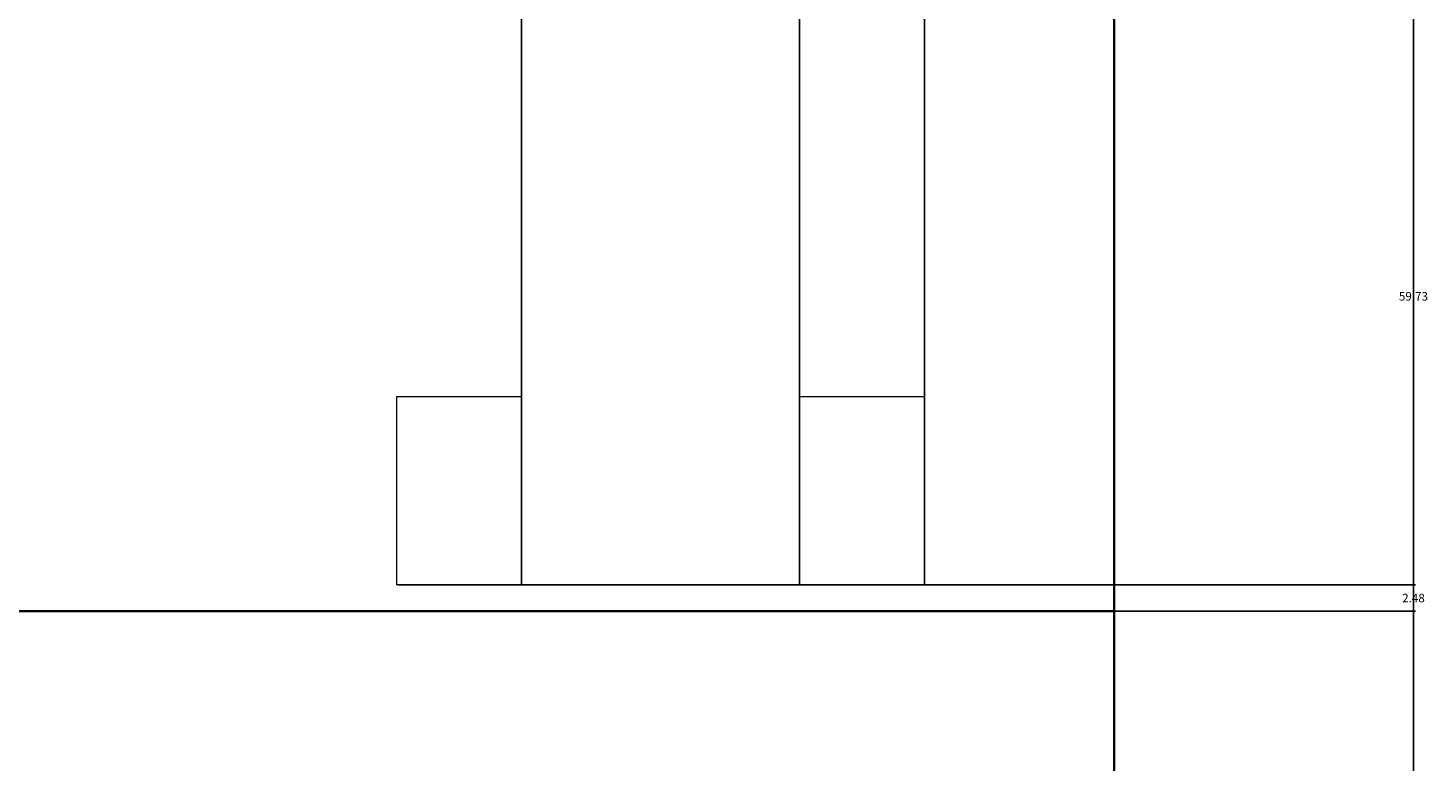
# Model space of a CAD drawing. Units: inches. Extents: x 69 to 650, y -16 to 573.
# Tile 25 of 26: x 516 to 649, y 398 to 467. Entities that reach past the tile are written whole.
import ezdxf

# ---------------------------------------------------------------- set-up
doc = ezdxf.new("R2010")
doc.units = ezdxf.units.IN
doc.header["$MEASUREMENT"] = 0
for name, color, linetype, lineweight in [('A-ANNO-DIMS', 2, 'Continuous', 18), ('A-GLAZ', 4, 'Continuous', 18), ('A-WALL', 7, 'Continuous', 35)]:
    doc.layers.add(name, color=color, linetype=linetype, lineweight=lineweight)
doc.styles.get("Standard").update_dxf_attribs({"font": 'arial.ttf'})
doc.dimstyles.get("Standard").update_dxf_attribs({"dimtxt": 0.8125, "dimasz": 0.18, "dimexe": 0.18, "dimexo": 0.0625, "dimgap": 0.09, "dimtad": 0, "dimtih": 1, "dimtoh": 1, "dimdec": 4, "dimzin": 0, "dimdsep": 46, "dimlunit": 4, "dimtxsty": 'Standard', "dimcen": 0.09, "dimadec": 0, "dimazin": 0, "dimtfac": 1, "dimtdec": 4, "dimtofl": 0, "dimtmove": 0, "dimatfit": 3, "dimfxl": 1, "dimtolj": 1, "dimtzin": 0, "dimarcsym": 0})

# ---------------------------------------------------------------- blocks, each defined once
blk = doc.blocks.new('WIN-UPPER-SMALL')
blk.add_lwpolyline([(0, 17.88), (11.84, 17.88), (11.84, 0), (0, 0)], close=True)
blk = doc.blocks.new('*D19')
at = {"layer": 'A-ANNO-DIMS', "color": 0, "lineweight": -2, "transparency": 16777216}
for p, q in [((99.56, 471.72), (99.56, 572.74)), ((619.56, 87.99), (619.56, 572.74)), ((99.74, 572.56), (358.57, 572.56)), ((619.38, 572.56), (360.54, 572.56))]:
    blk.add_line(p, q, dxfattribs=at)
at = {"layer": 'A-ANNO-DIMS', "color": 0, "transparency": 16777216}
for points in [[(99.74, 572.59), (99.74, 572.53), (99.56, 572.56)], [(619.38, 572.59), (619.38, 572.53), (619.56, 572.56)]]:
    blk.add_solid(points, dxfattribs=at)
at = {"layer": 'Defpoints', "color": 0, "transparency": 16777216}
for p in [(619.56, 572.56), (99.56, 471.66), (619.56, 87.93)]:
    blk.add_point(p, dxfattribs=at)
at = {"layer": 'A-ANNO-DIMS', "color": 0, "transparency": 16777216, "insert": (359.56, 572.56), "char_height": 0.812, "attachment_point": 5}
blk.add_mtext('\\A1;520', dxfattribs=at)
blk = doc.blocks.new('*D20')
at = {"layer": 'A-ANNO-DIMS', "color": 0, "lineweight": -2, "transparency": 16777216}
for p, q in [((504.24, 544.16), (648.14, 544.16)), ((647.96, 543.98), (647.96, 304.55)), ((647.96, 64.11), (647.96, 303.54)), ((619.62, 63.93), (648.14, 63.93))]:
    blk.add_line(p, q, dxfattribs=at)
at = {"layer": 'A-ANNO-DIMS', "color": 0, "transparency": 16777216}
for points in [[(647.93, 543.98), (647.99, 543.98), (647.96, 544.16)], [(647.93, 64.11), (647.99, 64.11), (647.96, 63.93)]]:
    blk.add_solid(points, dxfattribs=at)
at = {"layer": 'Defpoints', "color": 0, "transparency": 16777216}
for p in [(504.18, 544.16), (647.96, 544.16), (619.56, 63.93)]:
    blk.add_point(p, dxfattribs=at)
at = {"layer": 'A-ANNO-DIMS', "color": 0, "transparency": 16777216, "insert": (647.96, 304.04), "char_height": 0.812, "attachment_point": 5}
blk.add_mtext('\\A1;480.2', dxfattribs=at)
blk = doc.blocks.new('*D48')
at = {"layer": 'A-ANNO-DIMS', "color": 0, "lineweight": -2, "transparency": 16777216}
for p, q in [((619.62, 471.66), (648.14, 471.66)), ((647.96, 471.48), (647.96, 442.3)), ((647.96, 412.11), (647.96, 441.29)), ((619.62, 411.93), (648.14, 411.93))]:
    blk.add_line(p, q, dxfattribs=at)
at = {"layer": 'A-ANNO-DIMS', "color": 0, "transparency": 16777216}
for points in [[(647.93, 471.48), (647.99, 471.48), (647.96, 471.66)], [(647.93, 412.11), (647.99, 412.11), (647.96, 411.93)]]:
    blk.add_solid(points, dxfattribs=at)
at = {"layer": 'Defpoints', "color": 0, "transparency": 16777216}
for p in [(619.56, 471.66), (647.96, 471.66), (619.56, 411.93)]:
    blk.add_point(p, dxfattribs=at)
at = {"layer": 'A-ANNO-DIMS', "color": 0, "transparency": 16777216, "insert": (647.96, 441.79), "char_height": 0.812, "attachment_point": 5}
blk.add_mtext('\\A1;59.73', dxfattribs=at)
blk = doc.blocks.new('*D55')
at = {"layer": 'A-ANNO-DIMS', "color": 0, "lineweight": -2, "transparency": 16777216}
for p, q in [((563.31, 414.48), (563.31, 572.74)), ((589.7, 414.48), (589.7, 572.74)), ((563.49, 572.56), (575.03, 572.56)), ((589.52, 572.56), (577.97, 572.56))]:
    blk.add_line(p, q, dxfattribs=at)
at = {"layer": 'A-ANNO-DIMS', "color": 0, "transparency": 16777216}
for points in [[(563.49, 572.59), (563.49, 572.53), (563.31, 572.56)], [(589.52, 572.59), (589.52, 572.53), (589.7, 572.56)]]:
    blk.add_solid(points, dxfattribs=at)
at = {"layer": 'Defpoints', "color": 0, "transparency": 16777216}
for p in [(589.7, 572.56), (563.31, 414.41), (589.7, 414.41)]:
    blk.add_point(p, dxfattribs=at)
at = {"layer": 'A-ANNO-DIMS', "color": 0, "transparency": 16777216, "insert": (576.5, 572.56), "char_height": 0.812, "attachment_point": 5}
blk.add_mtext('\\A1;26.39', dxfattribs=at)
blk = doc.blocks.new('*D56')
at = {"layer": 'A-ANNO-DIMS', "color": 0, "lineweight": -2, "transparency": 16777216}
for p, q in [((601.54, 414.48), (601.54, 572.74)), ((619.56, 411.99), (619.56, 572.74)), ((601.72, 572.56), (608.81, 572.56)), ((619.38, 572.56), (612.29, 572.56))]:
    blk.add_line(p, q, dxfattribs=at)
at = {"layer": 'A-ANNO-DIMS', "color": 0, "transparency": 16777216}
for points in [[(601.72, 572.59), (601.72, 572.53), (601.54, 572.56)], [(619.38, 572.59), (619.38, 572.53), (619.56, 572.56)]]:
    blk.add_solid(points, dxfattribs=at)
at = {"layer": 'Defpoints', "color": 0, "transparency": 16777216}
for p in [(619.56, 572.56), (601.54, 414.41), (619.56, 411.93)]:
    blk.add_point(p, dxfattribs=at)
at = {"layer": 'A-ANNO-DIMS', "color": 0, "transparency": 16777216, "insert": (610.55, 572.56), "char_height": 0.812, "attachment_point": 5}
blk.add_mtext('\\A1;18.018', dxfattribs=at)
blk = doc.blocks.new('*D57')
at = {"layer": 'A-ANNO-DIMS', "color": 0, "lineweight": -2, "transparency": 16777216}
for p, q in [((551.53, 414.41), (648.14, 414.41)), ((647.96, 414.23), (647.96, 413.68)), ((500.33, 411.93), (648.14, 411.93)), ((647.96, 412.11), (647.96, 412.67))]:
    blk.add_line(p, q, dxfattribs=at)
at = {"layer": 'A-ANNO-DIMS', "color": 0, "transparency": 16777216}
for points in [[(647.93, 414.23), (647.99, 414.23), (647.96, 414.41)], [(647.93, 412.11), (647.99, 412.11), (647.96, 411.93)]]:
    blk.add_solid(points, dxfattribs=at)
at = {"layer": 'Defpoints', "color": 0, "transparency": 16777216}
for p in [(551.46, 414.41), (500.26, 411.93), (647.96, 411.93)]:
    blk.add_point(p, dxfattribs=at)
at = {"layer": 'A-ANNO-DIMS', "color": 0, "transparency": 16777216, "insert": (647.96, 413.17), "char_height": 0.812, "attachment_point": 5}
blk.add_mtext('\\A1;2.48', dxfattribs=at)

msp = doc.modelspace()

# ---------------------------------------------------------------- linework, layer by layer
at = {"layer": 'A-WALL'}
for p, q in [((619.555, 411.93), (619.555, 471.6595)), ((99.556, 411.93), (619.555, 411.93)), ((619.555, 411.93), (619.555, 69.3788))]:
    msp.add_line(p, q, dxfattribs=at)

# ---------------------------------------------------------------- block references
at = {"layer": 'A-GLAZ'}
for p in [(551.4642, 414.415), (589.6959, 414.415)]:
    msp.add_blockref('WIN-UPPER-SMALL', p, dxfattribs=at)

# ---------------------------------------------------------------- dimensions: what is measured, and where the dimension line sits
at = {"layer": 'A-ANNO-DIMS'}
for base, p1, p2, override, picture, middle in [((619.555, 572.5573), (99.556, 471.6595), (619.555, 87.93), {"dimdec": 0, "dimlfac": 1, "dimrnd": 0, "dimzin": 0, "dimdsep": 46, "dimlunit": 2}, '*D19', (359.5555, 572.5573)), ((589.6958, 572.5573), (563.3054, 414.4146), (589.6958, 414.4146), {"dimdec": 2, "dimlfac": 1, "dimrnd": 0, "dimzin": 0, "dimdsep": 46, "dimlunit": 2}, '*D55', (576.5006, 572.5573)), ((619.555, 572.5573), (601.5371, 414.4146), (619.555, 411.93), {"dimdec": 3, "dimlfac": 1, "dimrnd": 0, "dimzin": 0, "dimdsep": 46, "dimlunit": 2}, '*D56', (610.5461, 572.5573))]:
    dim = msp.add_linear_dim(base=base, p1=p1, p2=p2, dimstyle='Standard', override=override, dxfattribs=at)
    dim.commit()
    dim.dimension.update_dxf_attribs({"geometry": picture, "text_midpoint": middle})
for base, p1, p2, override, picture, middle in [((647.955, 544.1573), (619.555, 63.93), (504.1763, 544.1573), {"dimdec": 1, "dimlfac": 1, "dimrnd": 0, "dimzin": 0, "dimdsep": 46, "dimlunit": 2}, '*D20', (647.955, 304.0436)), ((647.955, 471.6595), (619.555, 411.93), (619.555, 471.6595), {"dimdec": 2, "dimlfac": 1, "dimrnd": 0, "dimzin": 0, "dimdsep": 46, "dimlunit": 2}, '*D48', (647.955, 441.7948)), ((647.955, 411.93), (551.4641, 414.4146), (500.263, 411.93), {"dimdec": 2, "dimlfac": 1, "dimrnd": 0, "dimzin": 0, "dimdsep": 46, "dimlunit": 2}, '*D57', (647.955, 413.1723))]:
    dim = msp.add_linear_dim(base=base, p1=p1, p2=p2, angle=90, dimstyle='Standard', override=override, dxfattribs=at)
    dim.commit()
    dim.dimension.update_dxf_attribs({"geometry": picture, "text_midpoint": middle})

doc.saveas('drawing.dxf')
